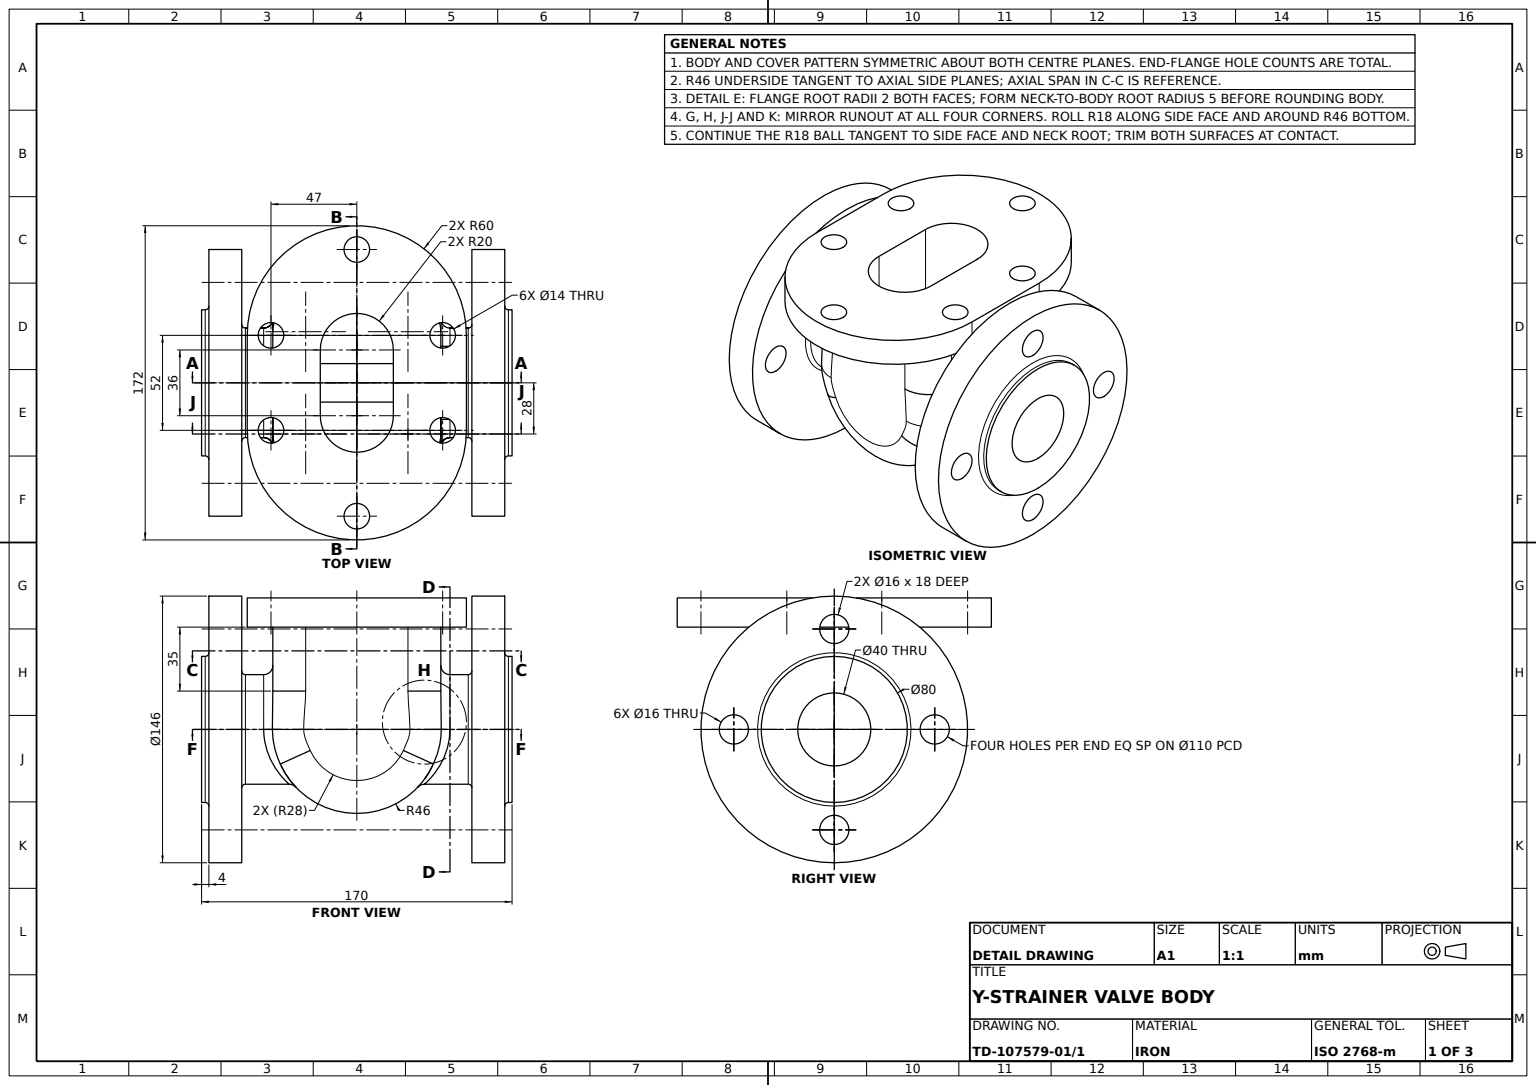
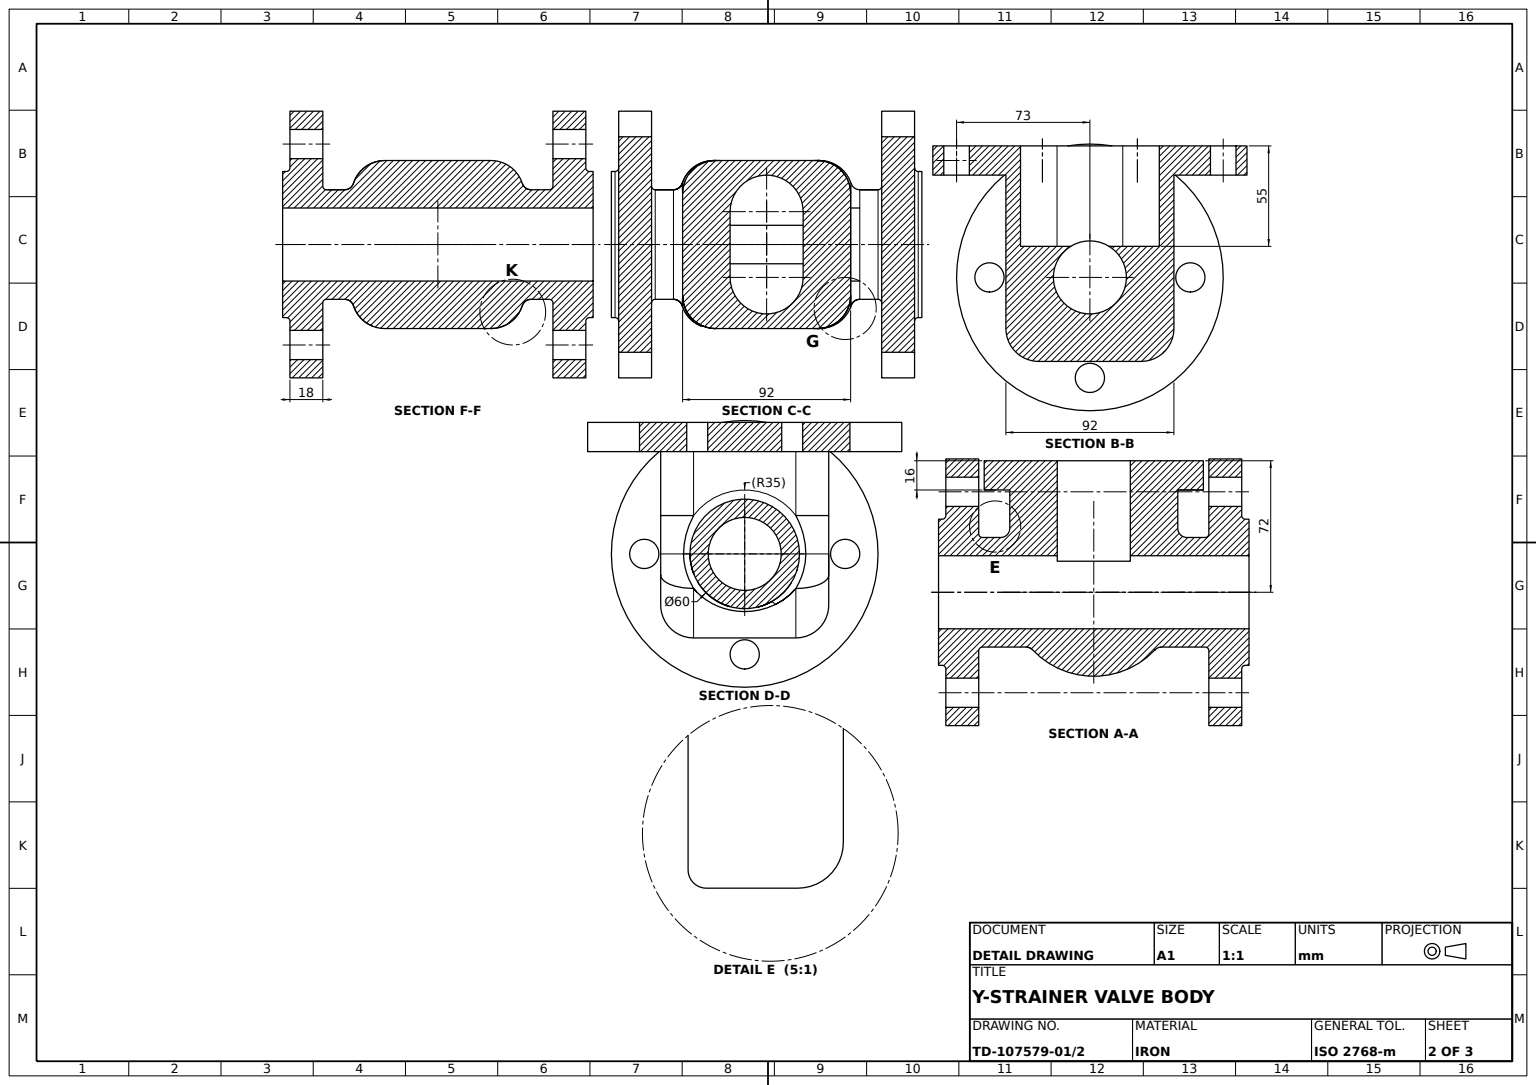
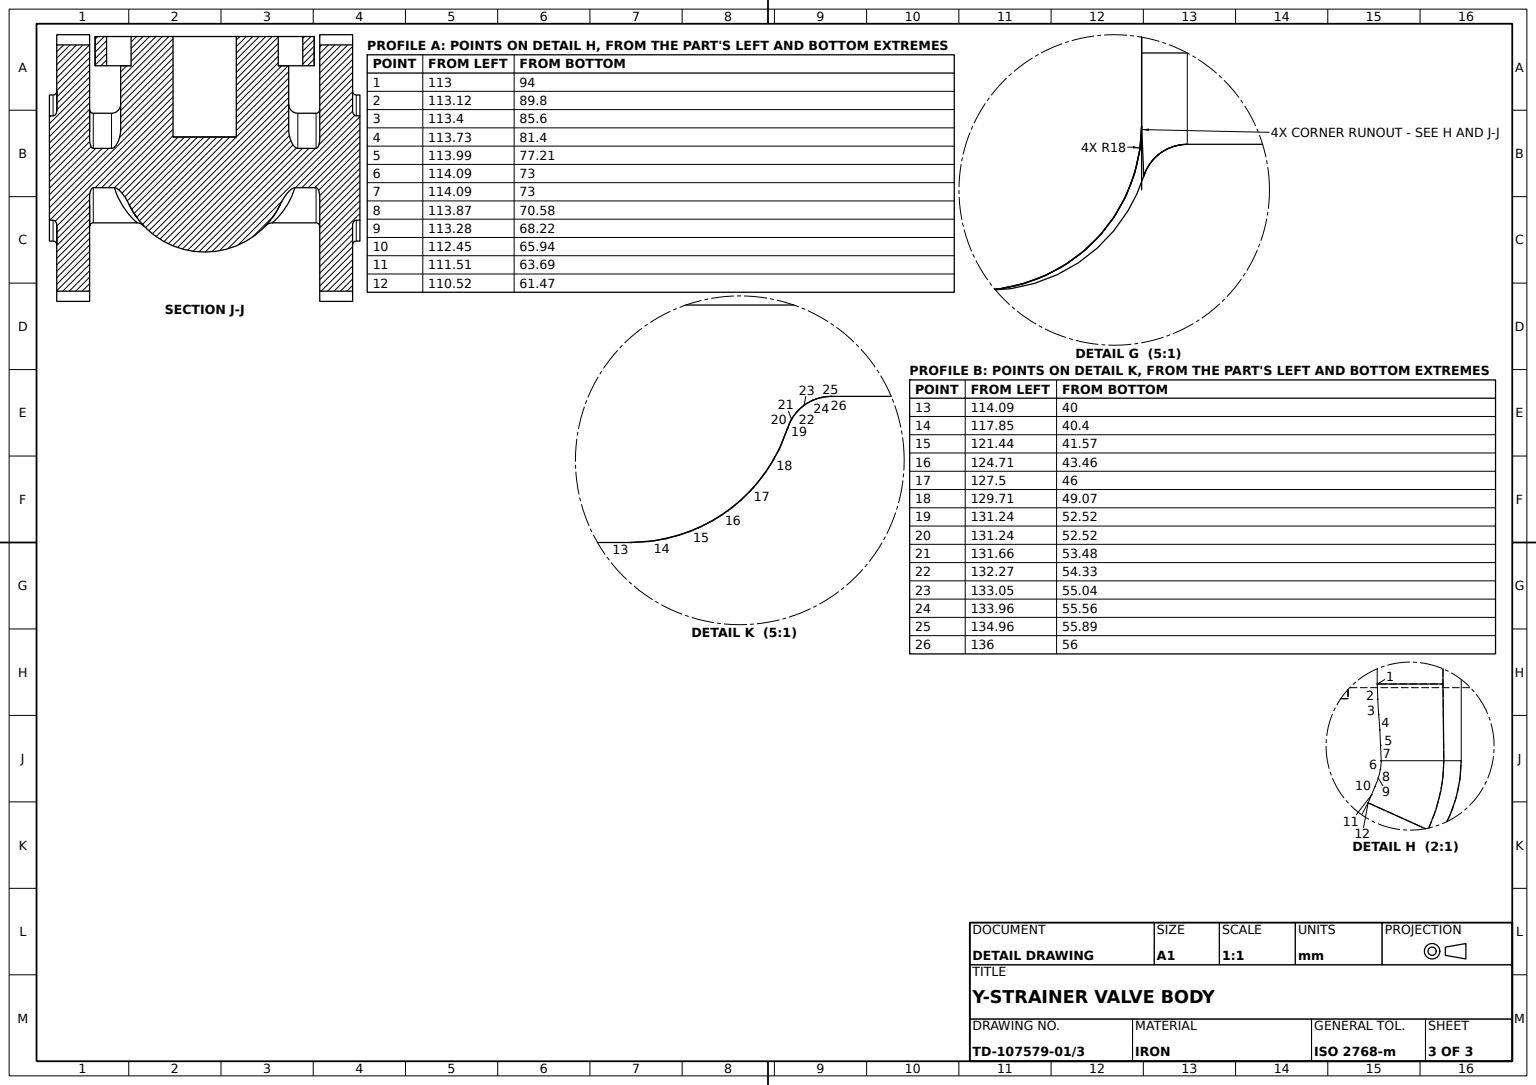
CATIA V5 part; units mm, degrees
sketch "Sketch1" plane through (0, 0, 0) normal (1, 0, 0) x (0, 1, 0)
  circle A0 centre (0, 0) radius 73
  dimension "radius A0" = 73
extrude "Pad1" add sketch "Sketch1" along normal blind 18
sketch "Sketch2" plane through (0, 0, 0) normal (0, 1, 0) x (-1, 0, 0)
  line L0 (0, 0) -> (-181.8709, 0) construction
  line L1 (-18, -30) -> (-144, -30)
  point P0 (-144, -30)
  line L2 (-18, 0) -> (-18, -30)
  point P1 (-144, -30)
  line L3 (-144, -30) -> (-144, 0)
  point P2 (-144, 0)
  line L4 (-144, 0) -> (-18, 0)
  line L5 (-18, -73) -> (-18, 73) construction
  dimension "length L3" = 30
  dimension "distance L3 L2" = 126
  constraint horizontal L0 x-axis
  constraint horizontal L1 x-axis
  constraint horizontal L4 x-axis
  constraint vertical L2 y-axis
  constraint vertical L3 y-axis
  constraint coincidence P2 L0
  constraint coincidence L5 L2
  constraint coincidence P0 P1
revolve "Shaft1" add sketch "Sketch2" angle 360 about L4
sketch "Sketch3" plane through (144, 0, 0) normal (1, 0, 0) x (0, 1, 0)
  circle A0 centre (0, 0) radius 73
extrude "Pad2" add sketch "Sketch3" along normal blind 18
sketch "Sketch4" plane through (162, 0, 0) normal (1, 0, 0) x (0, 1, 0)
  circle A0 centre (0, 0) radius 55 construction
  circle A1 centre (0, -55) radius 8
  point P0 (0, -55)
  dimension "radius A0" = 55
  dimension "radius A1" = 8
  constraint coincidence P0 A0
  constraint coincidence P0 y-axis
extrude "Pocket1" cut sketch "Sketch4" against normal through all
pattern_circular "CircPattern1" count 4 over 360 about axis through (162, 0, 0) along (1, 0, 0) of "Pocket1"
sketch "Sketch5" plane through (162, 0, 0) normal (1, 0, 0) x (0, 1, 0)
  circle A0 centre (0, 0) radius 40
  dimension "radius A0" = 40
extrude "Pad3" add sketch "Sketch5" along normal blind 4
sketch "Sketch6" plane through (0, 0, 0) normal (-1, 0, 0) x (0, -1, 0)
  circle A0 centre (0, 0) radius 40
  dimension "radius A0" = 40
extrude "Pad4" add sketch "Sketch6" along normal blind 4
fillet "Fillet1" radius 2 4 edges at (0, 40, 0) (144, 0, 30) (18, 0, 30) (162, -40, 0)
sketch "Sketch7" plane through (166, 0, 0) normal (1, 0, 0) x (0, 1, 0)
  circle A0 centre (0, 0) radius 20
  dimension "radius A0" = 20
extrude "Pocket2" cut sketch "Sketch7" against normal through all
ref_plane "Plane1" through (0, 0, 72) normal (0, 0, 1) x (1, 0, 0)
sketch "Sketch9" plane through (0, 0, 72) normal (0, 0, 1) x (0, 1, 0)
  point P0 (0, 0)
  line L0 (-26, -81) -> (26, -81) construction
  point P1 (-26, -81)
  point P2 (26, -81)
  line L1 (-26, -21) -> (26, -21)
  line L2 (26, -141) -> (-26, -141)
  arc A0 (26, -21) -> (26, -141) centre (26, -81) cw
  arc A1 (-26, -141) -> (-26, -21) centre (-26, -81) cw
  dimension "radius A0" = 60
  dimension "radius A1" = 60
  dimension "length L0" = 52
  dimension "distance P0 P2 y axis" = 81
  constraint horizontal L0 x-axis
  constraint tangency A0 L1
  constraint tangency A1 L1
  constraint tangency A0 L2
  constraint tangency A1 L2
  constraint coincidence P0 origin
  constraint symmetry P2 P1 y-axis
extrude "Pad5" add sketch "Sketch9" against normal blind 16
sketch "Sketch10" plane through (0, 0, 0) normal (0, 1, 0) x (-1, 0, 0)
  arc A0 (-127, 0) -> (-35, 0) centre (-81, 0) ccw
  point P0 (-81, 0)
  line L0 (0, -73) -> (0, 73) construction
  point P1 (-127, 0)
  line L1 (-127, 0) -> (-127, 56)
  point P2 (-35, 0)
  line L2 (-35, 0) -> (-35, 56)
  point P3 (-35, 56)
  line L3 (-35, 56) -> (-127, 56)
  point P4 (-127, 0)
  point P5 (-35, 0)
  line L4 (-55, 56) -> (-21, 56) construction
  dimension "radius A0" = 46
  dimension "distance P0 L0" = 81
  constraint coincidence P0 x-axis
  constraint coincidence P1 A0
  constraint coincidence P1 x-axis
  constraint coincidence P2 A0
  constraint coincidence P2 x-axis
  constraint coincidence L2 P5
  constraint coincidence L1 P4
  constraint coincidence P3 L4
  constraint coincidence P1 P4
  constraint coincidence P2 P5
  constraint tangency L1 A0
  constraint tangency L2 A0
  constraint horizontal L3 x-axis
extrude "Pad6" [suppressed]
fillet "Fillet2" [suppressed]
fillet "Fillet3" [suppressed]
fillet "Fillet4" [suppressed]
fillet "Fillet5" [suppressed]
fillet "Fillet6" [suppressed]
fillet "Fillet7" [suppressed]
fillet "Fillet8" [suppressed]
sketch "Sketch12" plane through (0, 0, 0) normal (0, 1, 0) x (-1, 0, 0)
  arc A0 (-127, 0) -> (-35, 0) centre (-81, 0) ccw
  point P0 (-81, 0)
  line L0 (-141, 56) -> (-21, 56) construction
  line L1 (-127, 56) -> (-35, 56)
  line L2 (-35, 0) -> (-35, 56)
  point P1 (-35, 0)
  point P2 (-35, 56)
  point P3 (-127, 0)
  line L3 (-127, 0) -> (-127, 56)
  point P4 (-127, 56)
  point P5 (-127, 0)
  point P6 (-35, 0)
  dimension "radius A0" = 46
  dimension "distance P0 origin" = 81
  constraint coincidence P0 x-axis
  constraint coincidence P1 A0
  constraint coincidence P1 x-axis
  constraint coincidence P2 L0
  constraint coincidence P3 A0
  constraint coincidence P3 x-axis
  constraint coincidence P4 L0
  constraint coincidence L2 P6
  constraint coincidence L3 P5
  constraint coincidence P1 P6
  constraint coincidence P3 P5
  constraint tangency L2 A0
  constraint tangency L3 A0
extrude "Pad7" add sketch "Sketch12" along normal mid plane 92
fillet "Fillet9" radius 5 2 edges at (40.2145, -21.1531, -21.2731) (40.2145, 21.1531, -21.2731)
fillet "Fillet10" radius 5 1 edges at (127, 0, 30)
fillet "Fillet11" radius 18 1 edges at (127, 46, 28)
fillet "Fillet12" radius 18 1 edges at (127, -46, 28)
sketch "Sketch13" plane through (0, 0, 72) normal (0, 0, 1) x (1, 0, 0)
  line L0 (81, 26) -> (81, -26) construction
  point P0 (81, 26)
  point P1 (81, -26)
  line L1 (128, 26) -> (128, -26) construction
  line L2 (34, -26) -> (34, 26) construction
  arc A0 (128, -26) -> (34, -26) centre (81, -26) cw construction
  arc A1 (34, 26) -> (128, 26) centre (81, 26) cw construction
  line L3 (0, 73) -> (0, -73) construction
  circle A2 centre (128, 26) radius 7
  circle A3 centre (128, -26) radius 7
  circle A4 centre (34, 26) radius 7
  circle A5 centre (34, -26) radius 7
  circle A6 centre (81, 73) radius 7
  point P2 (81, 73)
  circle A7 centre (81, -73) radius 7
  point P3 (81, -73)
  dimension "length L0" = 52
  dimension "radius A1" = 47
  dimension "radius A0" = 47
  dimension "distance L3 P1" = 81
  dimension "radius A2" = 7
  dimension "radius A3" = 7
  dimension "radius A5" = 7
  dimension "radius A4" = 7
  dimension "radius A7" = 7
  dimension "radius A6" = 7
  constraint vertical L0 y-axis
  constraint tangency A0 L1
  constraint tangency A1 L1
  constraint tangency A0 L2
  constraint tangency A1 L2
  constraint symmetry P1 P0 x-axis
  constraint coincidence P2 A1
  constraint coincidence P2 L0
  constraint coincidence P3 A0
  constraint coincidence P3 L0
extrude "Pocket3" cut sketch "Sketch13" against normal blind 16
sketch "Sketch14" plane through (0, 0, 72) normal (0, 0, 1) x (1, 0, 0)
  line L0 (81, 18) -> (81, -18) construction
  point P0 (81, 18)
  point P1 (81, -18)
  line L1 (101, 18) -> (101, -18)
  line L2 (61, -18) -> (61, 18)
  arc A0 (101, -18) -> (61, -18) centre (81, -18) cw
  arc A1 (61, 18) -> (101, 18) centre (81, 18) cw
  dimension "distance origin P1 x axis" = 81
  dimension "length L0" = 36
  dimension "radius A1" = 20
  dimension "radius A0" = 20
  constraint vertical L0 y-axis
  constraint tangency A0 L1
  constraint tangency A1 L1
  constraint tangency A0 L2
  constraint tangency A1 L2
  constraint symmetry P1 P0 x-axis
extrude "Pocket4" cut sketch "Sketch14" against normal blind 55
sketch "Sketch15" plane through (166, 0, 0) normal (1, 0, 0) x (0, 1, 0)
  circle A0 centre (0, 0) radius 20
extrude "Pocket5" cut sketch "Sketch15" against normal through all
sketch "Sketch8" plane through (0, 0, 72) normal (0, 0, 1) x (1, 0, 0)
sketch "Sketch11" plane through (0, 0, 72) normal (0, 0, 1) x (1, 0, 0)
equation "\"angular step@CircPattern1\" = 360.0*1 deg/CircPattern1.AngularNumber"
properties part number "Y-Strainer Valve Body" material "Iron"
